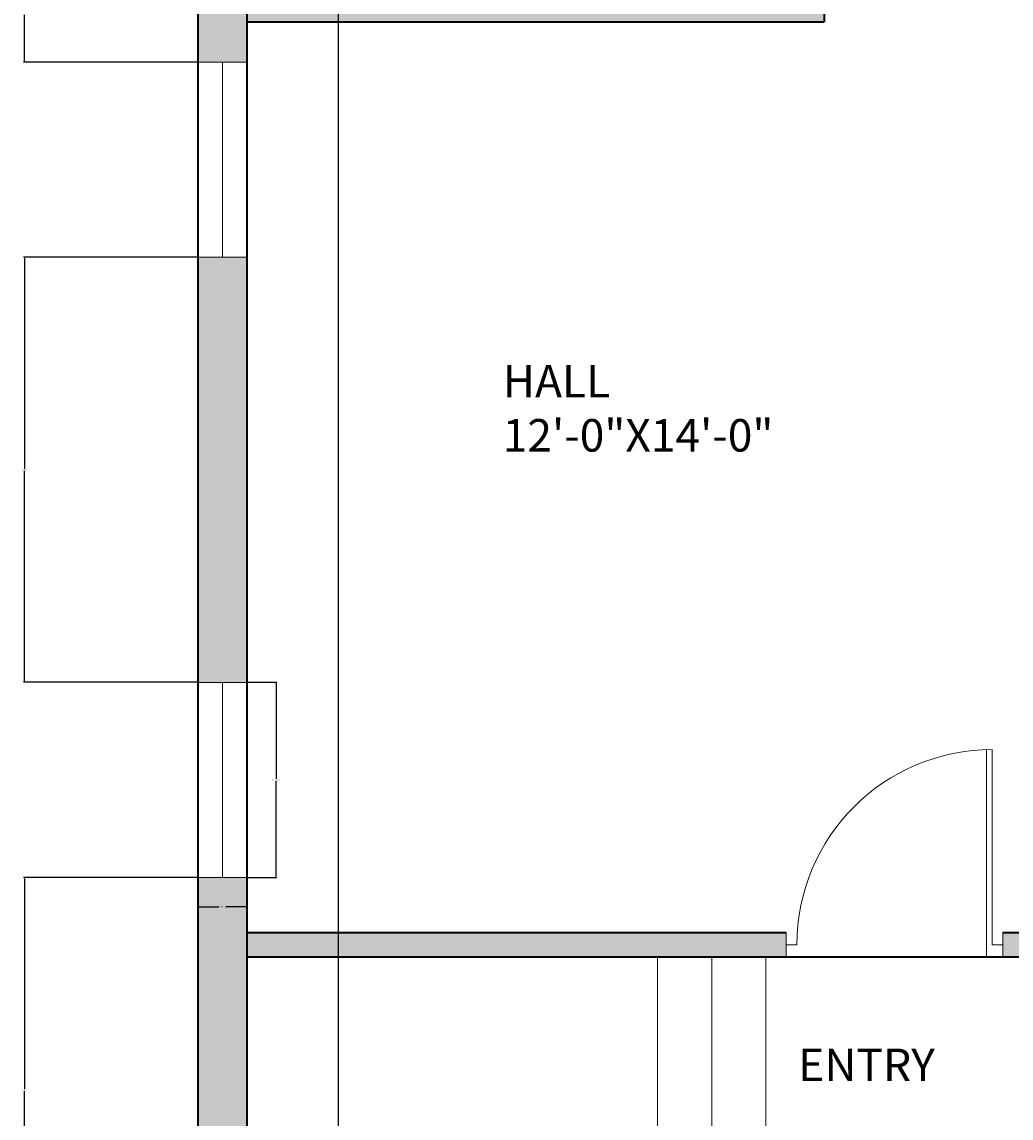
# Model space of a CAD drawing. Units: inches. Extents: x -13 to 349, y -556 to 61.
# Tile 2 of 6: x -13 to 170, y -351 to -149. Entities that reach past the tile are written whole.
import ezdxf

# ---------------------------------------------------------------- set-up
doc = ezdxf.new("R2010")
doc.units = ezdxf.units.IN
doc.header["$MEASUREMENT"] = 0
for name, color, linetype, lineweight in [('A-ANNO-DIMS', 2, 'Continuous', 18), ('A-AREA-IDEN', 7, 'Continuous', 18), ('A-DOOR', 3, 'Continuous', 20), ('A-FLOR-STRS', 7, 'Continuous', 20), ('A-GLAZ', 5, 'Continuous', 18), ('A-WALL', 7, 'Continuous', 35), ('A-WALL-PATT', 8, 'Continuous', 13)]:
    doc.layers.add(name, color=color, linetype=linetype, lineweight=lineweight)
doc.styles.get("Standard").update_dxf_attribs({"font": 'arial.ttf'})
doc.dimstyles.get("Standard").update_dxf_attribs({"dimtxt": 0.18, "dimasz": 0.18, "dimexe": 0.18, "dimexo": 0.0625, "dimgap": 0.09, "dimtad": 0, "dimtih": 1, "dimtoh": 1, "dimdec": 0, "dimzin": 0, "dimdsep": 46, "dimlunit": 3, "dimtxsty": 'Standard', "dimcen": 0.09, "dimadec": 0, "dimazin": 0, "dimtfac": 1, "dimtdec": 0, "dimtofl": 0, "dimtmove": 0, "dimatfit": 3, "dimfxl": 1, "dimtolj": 1, "dimtzin": 0, "dimarcsym": 0})

# ---------------------------------------------------------------- blocks, each defined once
blk = doc.blocks.new('DOOR-SWING-36IN')
for p, q in [((36, 40), (33.75, 40)), ((36, 38), (36, 40)), ((36, 40), (38.25, 40)), ((38.25, 3), (0, 3)), ((36, 2), (0, 2)), ((36, 0), (36, 2)), ((33.75, 0), (38.25, 0))]:
    blk.add_line(p, q)
blk.add_arc((36, 2), 36, 90, 180)
blk = doc.blocks.new('WIN-36IN-D9')
for p, q in [((0, 36), (0, 0)), ((9, 36), (0, 36)), ((4.5, 36), (4.5, 0)), ((9, 0), (9, 36)), ((0, 0), (9, 0))]:
    blk.add_line(p, q)
blk = doc.blocks.new('*D22')
at = {"layer": 'A-ANNO-DIMS', "color": 0, "lineweight": -2, "transparency": 16777216}
for p, q in [((28.82, -271.06), (34.34, -271.06)), ((34.16, -271.24), (34.16, -288.88)), ((34.16, -306.88), (34.16, -289.25)), ((28.82, -307.06), (34.34, -307.06))]:
    blk.add_line(p, q, dxfattribs=at)
at = {"layer": 'A-ANNO-DIMS', "color": 0, "transparency": 16777216}
for points in [[(34.13, -271.24), (34.19, -271.24), (34.16, -271.06)], [(34.13, -306.88), (34.19, -306.88), (34.16, -307.06)]]:
    blk.add_solid(points, dxfattribs=at)
at = {"layer": 'Defpoints', "color": 0, "transparency": 16777216}
for p in [(28.76, -271.06), (34.16, -271.06), (28.76, -307.06)]:
    blk.add_point(p, dxfattribs=at)
at = {"layer": 'A-ANNO-DIMS', "color": 0, "transparency": 16777216, "insert": (34.16, -289.06), "char_height": 0.18, "attachment_point": 5}
blk.add_mtext('\\A1;W3 3\'-0" TYP.', dxfattribs=at)
blk = doc.blocks.new('*D23')
at = {"layer": 'A-ANNO-DIMS', "color": 0, "lineweight": -2, "transparency": 16777216}
for p, q in [((19.76, -307.13), (19.76, -312.64)), ((28.76, -307.13), (28.76, -312.64)), ((19.94, -312.46), (23.62, -312.46)), ((28.58, -312.46), (24.89, -312.46))]:
    blk.add_line(p, q, dxfattribs=at)
at = {"layer": 'A-ANNO-DIMS', "color": 0, "transparency": 16777216}
for points in [[(19.94, -312.43), (19.94, -312.49), (19.76, -312.46)], [(28.58, -312.43), (28.58, -312.49), (28.76, -312.46)]]:
    blk.add_solid(points, dxfattribs=at)
at = {"layer": 'Defpoints', "color": 0, "transparency": 16777216}
for p in [(19.76, -307.06), (28.76, -307.06), (28.76, -312.46)]:
    blk.add_point(p, dxfattribs=at)
at = {"layer": 'A-ANNO-DIMS', "color": 0, "transparency": 16777216, "insert": (24.26, -312.46), "char_height": 0.18, "attachment_point": 5}
blk.add_mtext('\\A1;0\'-9" TYP.', dxfattribs=at)
blk = doc.blocks.new('*D38')
at = {"layer": 'A-ANNO-DIMS', "color": 0, "lineweight": -2, "transparency": 16777216}
for p, q in [((28.76, -144.78), (28.76, -555.89)), ((45.63, -144.78), (45.63, -555.89)), ((28.94, -555.71), (36.87, -555.71)), ((45.45, -555.71), (37.51, -555.71))]:
    blk.add_line(p, q, dxfattribs=at)
at = {"layer": 'A-ANNO-DIMS', "color": 0, "transparency": 16777216}
for points in [[(28.94, -555.68), (28.94, -555.74), (28.76, -555.71)], [(45.45, -555.68), (45.45, -555.74), (45.63, -555.71)]]:
    blk.add_solid(points, dxfattribs=at)
at = {"layer": 'Defpoints', "color": 0, "transparency": 16777216}
for p in [(28.76, -144.71), (45.63, -144.71), (45.63, -555.71)]:
    blk.add_point(p, dxfattribs=at)
at = {"layer": 'A-ANNO-DIMS', "color": 0, "transparency": 16777216, "insert": (37.19, -555.71), "char_height": 0.18, "attachment_point": 5}
blk.add_mtext('\\A1;1\'-5"', dxfattribs=at)
blk = doc.blocks.new('*D44')
at = {"layer": 'A-ANNO-DIMS', "color": 0, "lineweight": -2, "transparency": 16777216}
for p, q in [((19.69, -138.88), (-12.42, -138.88)), ((-12.24, -139.06), (-12.24, -147.56)), ((-12.24, -156.44), (-12.24, -147.93)), ((19.69, -156.62), (-12.42, -156.62))]:
    blk.add_line(p, q, dxfattribs=at)
at = {"layer": 'A-ANNO-DIMS', "color": 0, "transparency": 16777216}
for points in [[(-12.27, -139.06), (-12.21, -139.06), (-12.24, -138.88)], [(-12.27, -156.44), (-12.21, -156.44), (-12.24, -156.62)]]:
    blk.add_solid(points, dxfattribs=at)
at = {"layer": 'Defpoints', "color": 0, "transparency": 16777216}
for p in [(19.76, -138.88), (-12.24, -156.62), (19.76, -156.62)]:
    blk.add_point(p, dxfattribs=at)
at = {"layer": 'A-ANNO-DIMS', "color": 0, "transparency": 16777216, "insert": (-12.24, -147.75), "char_height": 0.18, "attachment_point": 5}
blk.add_mtext('\\A1;1\'-5 1/2"', dxfattribs=at)
blk = doc.blocks.new('*D45')
at = {"layer": 'A-ANNO-DIMS', "color": 0, "lineweight": -2, "transparency": 16777216}
for p, q in [((19.69, -192.62), (-12.42, -192.62)), ((-12.24, -192.8), (-12.24, -231.66)), ((-12.24, -270.88), (-12.24, -232.02)), ((19.69, -271.06), (-12.42, -271.06))]:
    blk.add_line(p, q, dxfattribs=at)
at = {"layer": 'A-ANNO-DIMS', "color": 0, "transparency": 16777216}
for points in [[(-12.27, -192.8), (-12.21, -192.8), (-12.24, -192.62)], [(-12.27, -270.88), (-12.21, -270.88), (-12.24, -271.06)]]:
    blk.add_solid(points, dxfattribs=at)
at = {"layer": 'Defpoints', "color": 0, "transparency": 16777216}
for p in [(19.76, -192.62), (-12.24, -271.06), (19.76, -271.06)]:
    blk.add_point(p, dxfattribs=at)
at = {"layer": 'A-ANNO-DIMS', "color": 0, "transparency": 16777216, "insert": (-12.24, -231.84), "char_height": 0.18, "attachment_point": 5}
blk.add_mtext('\\A1;6\'-6 1/2"', dxfattribs=at)
blk = doc.blocks.new('*D46')
at = {"layer": 'A-ANNO-DIMS', "color": 0, "lineweight": -2, "transparency": 16777216}
for p, q in [((19.69, -307.06), (-12.42, -307.06)), ((-12.24, -307.24), (-12.24, -346.13)), ((-12.24, -385.38), (-12.24, -346.49)), ((19.69, -385.56), (-12.42, -385.56))]:
    blk.add_line(p, q, dxfattribs=at)
at = {"layer": 'A-ANNO-DIMS', "color": 0, "transparency": 16777216}
for points in [[(-12.27, -307.24), (-12.21, -307.24), (-12.24, -307.06)], [(-12.27, -385.38), (-12.21, -385.38), (-12.24, -385.56)]]:
    blk.add_solid(points, dxfattribs=at)
at = {"layer": 'Defpoints', "color": 0, "transparency": 16777216}
for p in [(19.76, -307.06), (-12.24, -385.56), (19.76, -385.56)]:
    blk.add_point(p, dxfattribs=at)
at = {"layer": 'A-ANNO-DIMS', "color": 0, "transparency": 16777216, "insert": (-12.24, -346.31), "char_height": 0.18, "attachment_point": 5}
blk.add_mtext('\\A1;6\'-6 1/2"', dxfattribs=at)

msp = doc.modelspace()

# ---------------------------------------------------------------- hatches: boundary and pattern name
at = {"layer": 'A-WALL-PATT'}
h = msp.add_hatch(color=256, dxfattribs=at)
h.dxf.hatch_style = 1
h.paths.add_polyline_path([(316.76, 8.29), (171.26, 8.29), (171.26, -0.71), (307.76, -0.71), (307.76, -52.19), (316.76, -52.19)])
h.paths.add_polyline_path([(175.76, -0.71), (171.26, -0.71), (171.26, -82.21), (165.24, -82.21), (165.24, -86.71), (171.26, -86.71), (171.26, -101.71), (173.51, -101.71), (175.76, -101.71)])
h.paths.add_polyline_path([(171.26, -25.21), (165.17, -25.21), (165.17, -34.21), (171.26, -34.21)])
h.paths.add_polyline_path([(141.17, -25.21), (127.76, -25.21), (127.76, -34.21), (141.17, -34.21)])
h.paths.add_polyline_path([(28.76, -25.21), (24.26, -25.21), (19.76, -25.21), (19.76, -78.88), (28.76, -78.88)])
h.paths.add_polyline_path([(99.76, -29.71), (99.76, -25.21), (28.76, -25.21), (28.76, -34.21), (99.76, -34.21)])
h.paths.add_polyline_path([(135.26, -86.71), (143.68, -86.71), (143.68, -82.21), (135.26, -82.21), (135.26, -34.21), (130.76, -34.21), (130.76, -101.71), (133.01, -101.71), (135.26, -101.71)])
h.paths.add_polyline_path([(135.26, -141.71), (130.76, -141.71), (130.76, -144.71), (28.76, -144.71), (28.76, -149.21), (135.26, -149.21)])
h.paths.add_polyline_path([(28.76, -138.88), (19.76, -138.88), (19.76, -156.62), (28.76, -156.62)])
h.paths.add_polyline_path([(28.76, -192.62), (19.76, -192.62), (19.76, -271.06), (28.76, -271.06)])
h.paths.add_polyline_path([(28.76, -307.06), (19.76, -307.06), (19.76, -385.56), (28.76, -385.56)])
h.paths.add_polyline_path([(28.76, -445.56), (19.76, -445.56), (19.76, -523.71), (28.76, -523.71)])
h.paths.add_polyline_path([(307.76, -431.71), (261.76, -431.71), (261.76, -353.71), (264.76, -353.71), (264.76, -349.21), (175.76, -349.21), (175.76, -248.21), (173.51, -248.21), (171.26, -248.21), (171.26, -317.21), (168.26, -317.21), (168.26, -321.71), (171.26, -321.71), (171.26, -353.71), (257.26, -353.71), (257.26, -431.71), (171.26, -431.71), (171.26, -436.21), (307.76, -436.21)])
h.paths.add_polyline_path([(316.76, -424.85), (307.76, -424.85), (307.76, -436.21), (316.76, -436.21)])
h.paths.add_polyline_path([(316.76, -305.84), (307.76, -305.84), (307.76, -400.85), (316.76, -400.85)])
h.paths.add_polyline_path([(307.76, -349.21), (292.76, -349.21), (292.76, -351.46), (292.76, -353.71), (307.76, -353.71)], flags=17)
h.paths.add_polyline_path([(271.19, -200.71), (267.26, -200.71), (267.26, -186.96), (262.76, -186.96), (262.76, -200.71), (175.76, -200.71), (175.76, -180.21), (173.51, -180.21), (171.26, -180.21), (171.26, -208.21), (175.76, -208.21), (175.76, -205.21), (271.19, -205.21)])
h.paths.add_polyline_path([(316.76, -112.19), (307.76, -112.19), (307.76, -245.84), (316.76, -245.84)])
h.paths.add_polyline_path([(271.33, -144.71), (175.76, -144.71), (175.76, -141.71), (171.26, -141.71), (171.26, -152.21), (175.76, -152.21), (175.76, -149.21), (262.76, -149.21), (262.76, -162.96), (267.26, -162.96), (267.26, -149.21), (271.33, -149.21)])
h.paths.add_polyline_path([(307.76, -200.71), (307.19, -200.71), (307.19, -205.21), (307.76, -205.21)])
h.paths.add_polyline_path([(307.76, -144.71), (307.33, -144.71), (307.33, -149.21), (307.76, -149.21)])
h = msp.add_hatch(color=256, dxfattribs=at)
h.dxf.hatch_style = 1
h.paths.add_polyline_path([(128.26, -317.21), (28.76, -317.21), (28.76, -321.71), (128.26, -321.71), (128.26, -319.46)])

# ---------------------------------------------------------------- linework, layer by layer
at = {"layer": 'A-FLOR-STRS'}
for p, q in [((104.53, -353.71), (104.53, -321.71)), ((114.53, -353.71), (114.53, -321.71)), ((124.53, -321.71), (124.53, -353.71))]:
    msp.add_line(p, q, dxfattribs=at)
at = {"layer": 'A-WALL'}
for p, q in [((19.76, 8.29), (19.76, -523.71)), ((28.76, -25.21), (28.76, -523.71)), ((135.26, -86.71), (135.26, -149.21)), ((28.76, -149.21), (135.26, -149.21)), ((28.76, -317.21), (128.26, -317.21)), ((168.26, -317.21), (171.26, -317.21)), ((28.76, -321.71), (171.26, -321.71))]:
    msp.add_line(p, q, dxfattribs=at)

# ---------------------------------------------------------------- block references
at = {"layer": 'A-DOOR', "extrusion": (0, 0, -1), "zscale": -1, "rotation": 270.0000000000001}
msp.add_blockref('DOOR-SWING-36IN', (-168.25, -283.47), dxfattribs=at)
at = {"layer": 'A-GLAZ'}
for p in [(19.76, -192.62), (19.76, -307.07)]:
    msp.add_blockref('WIN-36IN-D9', p, dxfattribs=at)

# ---------------------------------------------------------------- texts
at = {"layer": 'A-AREA-IDEN', "char_height": 6, "attachment_point": 1}
for s, insert in [('HALL\\P12\'-0"X14\'-0"', (75.98, -212.49)), ('ENTRY', (130.49, -338.65))]:
    msp.add_mtext(s, dxfattribs=dict(at, insert=insert))

# ---------------------------------------------------------------- dimensions: what is measured, and where the dimension line sits
at = {"layer": 'A-ANNO-DIMS'}
for base, p1, p2, picture, middle in [((-12.24, -156.62), (19.76, -138.88), (19.76, -156.62), '*D44', (-12.24, -147.75)), ((-12.24, -271.06), (19.76, -192.62), (19.76, -271.06), '*D45', (-12.24, -231.84)), ((-12.24, -385.56), (19.76, -307.06), (19.76, -385.56), '*D46', (-12.24, -346.31))]:
    dim = msp.add_linear_dim(base=base, p1=p1, p2=p2, angle=90, dimstyle='Standard', override={"dimdec": 1, "dimlfac": 1, "dimrnd": 0, "dimzin": 1, "dimdsep": 46, "dimlunit": 4, "dimfrac": 2}, dxfattribs=at)
    dim.commit()
    dim.dimension.update_dxf_attribs({"geometry": picture, "text_midpoint": middle})
dim = msp.add_linear_dim(base=(45.63, -555.71), p1=(28.76, -144.71), p2=(45.63, -144.71), dimstyle='Standard', override={"dimdec": 1, "dimlfac": 1, "dimrnd": 0, "dimzin": 1, "dimdsep": 46, "dimlunit": 4, "dimfrac": 2}, dxfattribs=at)
dim.commit()
dim.dimension.update_dxf_attribs({"geometry": '*D38', "text_midpoint": (37.19, -555.71)})
dim = msp.add_linear_dim(base=(34.16, -271.06), p1=(28.76, -307.06), p2=(28.76, -271.06), angle=90, text='W3 <> TYP.', dimstyle='Standard', override={"dimdec": 1, "dimlfac": 1, "dimrnd": 0, "dimzin": 1, "dimdsep": 46, "dimlunit": 4, "dimfrac": 2}, dxfattribs=at)
dim.commit()
dim.dimension.update_dxf_attribs({"geometry": '*D22', "text_midpoint": (34.16, -289.06)})
dim = msp.add_linear_dim(base=(28.76, -312.46), p1=(19.76, -307.06), p2=(28.76, -307.06), text='<> TYP.', dimstyle='Standard', override={"dimdec": 1, "dimlfac": 1, "dimrnd": 0, "dimzin": 1, "dimdsep": 46, "dimlunit": 4, "dimfrac": 2}, dxfattribs=at)
dim.commit()
dim.dimension.update_dxf_attribs({"geometry": '*D23', "text_midpoint": (24.26, -312.46)})

doc.saveas('drawing.dxf')
